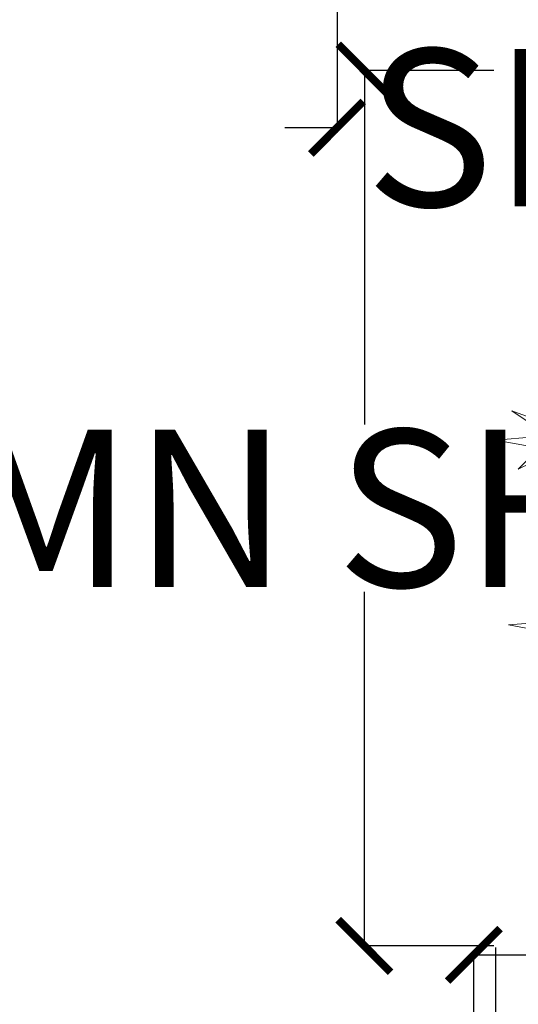
# Model space of a CAD drawing. Units: inches. Extents: x 1704 to 6393, y -157 to 1172.
# Tile 11 of 122: x 1879 to 1898, y 120 to 157. Entities that reach past the tile are written whole.
import ezdxf

# ---------------------------------------------------------------- set-up
doc = ezdxf.new("R2010")
doc.units = ezdxf.units.IN
doc.header["$MEASUREMENT"] = 0
doc.layers.add('A-ANNO-DIMS', color=7, linetype='Continuous', lineweight=13)
doc.layers.add('L-shrub', color=74, linetype='Continuous', lineweight=18)
doc.styles.get("Standard").update_dxf_attribs({"font": 'arial.ttf'})
doc.dimstyles.get("Standard").update_dxf_attribs({"dimtxt": 6, "dimasz": 2, "dimexe": 0.18, "dimexo": 0.0625, "dimgap": 0.09, "dimtad": 0, "dimtih": 1, "dimtoh": 1, "dimdec": 1, "dimzin": 0, "dimdsep": 46, "dimlunit": 3, "dimtxsty": 'Standard', "dimblk": 'ARCHTICK', "dimcen": 0.09, "dimadec": 0, "dimazin": 0, "dimtfac": 1, "dimtdec": 1, "dimtofl": 0, "dimtmove": 0, "dimatfit": 3, "dimfxl": 1, "dimtolj": 1, "dimtzin": 0, "dimarcsym": 0})

# ---------------------------------------------------------------- blocks, each defined once
blk = doc.blocks.new('autumn shrub')
at = {"layer": 'L-shrub'}
for points in [[(-46.17, -236.34), (-38.48, -236.34), (-53.87, -259.4), (-46.17, -238.26)], [(69.26, -238.26), (76.95, -240.18), (73.11, -261.32), (71.18, -238.26)], [(-32.71, -242.11), (-19.24, -255.56), (-26.93, -240.18), (-30.78, -242.11)], [(-40.4, -245.95), (-32.71, -247.87), (-36.55, -269.01), (-38.48, -245.95)]]:
    blk.add_lwpolyline(points, dxfattribs=at)
blk = doc.blocks.new('_ArchTick')
at = {"color": 0, "linetype": 'ByBlock', "const_width": 0.15}
blk.add_lwpolyline([(-0.5, -0.5), (0.5, 0.5)], dxfattribs=at)
blk = doc.blocks.new('*D74')
at = {"layer": 'A-ANNO-DIMS', "color": 0, "lineweight": -2, "transparency": 16777216}
for p, q in [((1890.878, 159.062), (1890.878, 152.884)), ((1931.278, 159.062), (1931.278, 152.884)), ((1890.878, 153.064), (1888.878, 153.064)), ((1931.278, 153.064), (1933.278, 153.064))]:
    blk.add_line(p, q, dxfattribs=at)
at = {"layer": 'Defpoints', "color": 0, "lineweight": -3, "transparency": 16777216}
for p in [(1890.878, 159.124), (1931.278, 159.124), (1931.278, 153.064)]:
    blk.add_point(p, dxfattribs=at)
at = {"layer": 'A-ANNO-DIMS', "color": 0, "lineweight": -2, "transparency": 16777216, "xscale": 2, "yscale": 2, "zscale": 2}
blk.add_blockref('_ArchTick', (1890.878, 153.064), dxfattribs=at)
at = {"layer": 'A-ANNO-DIMS', "color": 0, "lineweight": -2, "transparency": 16777216, "xscale": 2, "yscale": 2, "zscale": 2, "rotation": 180}
blk.add_blockref('_ArchTick', (1931.278, 153.064), dxfattribs=at)
at = {"layer": 'A-ANNO-DIMS', "color": 0, "transparency": 16777216, "insert": (1911.078, 153.064), "char_height": 6, "attachment_point": 5}
blk.add_mtext('\\A1;SHRUB 40', dxfattribs=at)
blk = doc.blocks.new('*D78')
at = {"layer": 'A-ANNO-DIMS', "color": 0, "lineweight": -2, "transparency": 16777216}
for p, q in [((1896.87, 155.246), (1891.743, 155.246)), ((1891.923, 155.246), (1891.923, 141.742)), ((1891.923, 121.849), (1891.923, 135.353)), ((1896.87, 121.849), (1891.743, 121.849))]:
    blk.add_line(p, q, dxfattribs=at)
at = {"layer": 'Defpoints', "color": 0, "lineweight": -3, "transparency": 16777216}
for p in [(1896.932, 155.246), (1891.923, 121.849), (1896.932, 121.849)]:
    blk.add_point(p, dxfattribs=at)
at = {"layer": 'A-ANNO-DIMS', "color": 0, "lineweight": -2, "transparency": 16777216, "xscale": 2, "yscale": 2, "zscale": 2}
for p, rotation in [((1891.923, 155.246), 90), ((1891.923, 121.849), 270)]:
    blk.add_blockref('_ArchTick', p, dxfattribs=dict(at, rotation=rotation))
at = {"layer": 'A-ANNO-DIMS', "color": 0, "transparency": 16777216, "insert": (1891.923, 138.547), "char_height": 6, "attachment_point": 5}
blk.add_mtext('\\A1;AUTUMN SHRUB 33', dxfattribs=at)
blk = doc.blocks.new('*D79')
at = {"layer": 'A-ANNO-DIMS', "color": 0, "lineweight": -2, "transparency": 16777216}
for p, q in [((1896.932, 121.786), (1896.932, 116.659)), ((1930.289, 121.786), (1930.289, 116.659)), ((1896.932, 116.839), (1909.225, 116.839)), ((1930.289, 116.839), (1917.996, 116.839))]:
    blk.add_line(p, q, dxfattribs=at)
at = {"layer": 'Defpoints', "color": 0, "lineweight": -3, "transparency": 16777216}
for p in [(1896.932, 121.849), (1930.289, 121.849), (1930.289, 116.839)]:
    blk.add_point(p, dxfattribs=at)
at = {"layer": 'A-ANNO-DIMS', "color": 0, "lineweight": -2, "transparency": 16777216, "xscale": 2, "yscale": 2, "zscale": 2, "rotation": 180}
blk.add_blockref('_ArchTick', (1896.932, 116.839), dxfattribs=at)
at = {"layer": 'A-ANNO-DIMS', "color": 0, "lineweight": -2, "transparency": 16777216, "xscale": 2, "yscale": 2, "zscale": 2}
blk.add_blockref('_ArchTick', (1930.289, 116.839), dxfattribs=at)
at = {"layer": 'A-ANNO-DIMS', "color": 0, "transparency": 16777216, "insert": (1913.611, 116.839), "char_height": 6, "attachment_point": 5}
blk.add_mtext('\\A1;33', dxfattribs=at)
blk = doc.blocks.new('*D83')
at = {"layer": 'A-ANNO-DIMS', "color": 0, "lineweight": -2, "transparency": 16777216}
for p, q in [((1896.102, 116.575), (1896.102, 121.691)), ((1896.102, 121.511), (1907.632, 121.511)), ((1927.871, 121.511), (1916.342, 121.511)), ((1927.871, 116.575), (1927.871, 121.691))]:
    blk.add_line(p, q, dxfattribs=at)
at = {"layer": 'Defpoints', "color": 0, "lineweight": -3, "transparency": 16777216}
for p in [(1927.871, 121.511), (1896.102, 116.512), (1927.871, 116.512)]:
    blk.add_point(p, dxfattribs=at)
at = {"layer": 'A-ANNO-DIMS', "color": 0, "lineweight": -2, "transparency": 16777216, "xscale": 2, "yscale": 2, "zscale": 2, "rotation": 180}
blk.add_blockref('_ArchTick', (1896.102, 121.511), dxfattribs=at)
at = {"layer": 'A-ANNO-DIMS', "color": 0, "lineweight": -2, "transparency": 16777216, "xscale": 2, "yscale": 2, "zscale": 2}
blk.add_blockref('_ArchTick', (1927.871, 121.511), dxfattribs=at)
at = {"layer": 'A-ANNO-DIMS', "color": 0, "transparency": 16777216, "insert": (1911.987, 121.511), "char_height": 6, "attachment_point": 5}
blk.add_mtext('\\A1;32', dxfattribs=at)
blk = doc.blocks.new('*D93')
at = {"layer": 'A-ANNO-DIMS', "color": 0, "lineweight": -2, "transparency": 16777216}
for p, q in [((2605.286, 895.213), (1829.698, 895.213)), ((1829.878, 895.213), (1829.878, 495.866)), ((1829.878, 90.213), (1829.878, 489.56)), ((2605.286, 90.213), (1829.698, 90.213))]:
    blk.add_line(p, q, dxfattribs=at)
at = {"layer": 'Defpoints', "color": 0, "lineweight": -3, "transparency": 16777216}
for p in [(2605.349, 895.213), (1829.878, 90.213), (2605.349, 90.213)]:
    blk.add_point(p, dxfattribs=at)
at = {"layer": 'A-ANNO-DIMS', "color": 0, "lineweight": -2, "transparency": 16777216, "xscale": 2, "yscale": 2, "zscale": 2}
for p, rotation in [((1829.878, 895.213), 90), ((1829.878, 90.213), 270)]:
    blk.add_blockref('_ArchTick', p, dxfattribs=dict(at, rotation=rotation))
at = {"layer": 'A-ANNO-DIMS', "color": 0, "transparency": 16777216, "insert": (1829.878, 492.713), "char_height": 6, "attachment_point": 5}
blk.add_mtext('\\A1;805', dxfattribs=at)

msp = doc.modelspace()

# ---------------------------------------------------------------- block references
at = {"layer": 'L-shrub', "xscale": 0.0642956299502212, "yscale": 0.0642956299502212, "zscale": 0.0642956299502212, "rotation": 270}
msp.add_blockref('autumn shrub', (1914.228, 138.795), dxfattribs=at)

# ---------------------------------------------------------------- dimensions: what is measured, and where the dimension line sits
at = {"layer": 'A-ANNO-DIMS'}
dim = msp.add_linear_dim(base=(1829.878, 90.213), p1=(2605.349, 895.213), p2=(2605.349, 90.213), angle=90, dimstyle='Standard', override={"dimdec": 0, "dimlfac": 1, "dimrnd": 0, "dimzin": 0, "dimdsep": 46, "dimlunit": 2}, dxfattribs=at)
dim.commit()
dim.dimension.update_dxf_attribs({"geometry": '*D93', "text_midpoint": (1829.878, 492.713)})
dim = msp.add_linear_dim(base=(1931.278, 153.064), p1=(1890.878, 159.124), p2=(1931.278, 159.124), text='SHRUB <>', dimstyle='Standard', override={"dimdec": 0, "dimlfac": 1, "dimrnd": 0, "dimzin": 0, "dimdsep": 46, "dimlunit": 2}, dxfattribs=at)
dim.commit()
dim.dimension.update_dxf_attribs({"geometry": '*D74', "text_midpoint": (1911.078, 153.064)})
dim = msp.add_linear_dim(base=(1891.923, 121.849), p1=(1896.932, 155.246), p2=(1896.932, 121.849), angle=270, text='AUTUMN SHRUB <>', dimstyle='Standard', override={"dimdec": 0, "dimlfac": 1, "dimrnd": 0, "dimzin": 0, "dimdsep": 46, "dimlunit": 2}, dxfattribs=at)
dim.commit()
dim.dimension.update_dxf_attribs({"geometry": '*D78', "text_midpoint": (1891.923, 138.547)})
for base, p1, p2, picture, middle in [((1927.871, 121.511), (1896.102, 116.512), (1927.871, 116.512), '*D83', (1911.987, 121.511)), ((1930.289, 116.839), (1896.932, 121.849), (1930.289, 121.849), '*D79', (1913.611, 116.839))]:
    dim = msp.add_linear_dim(base=base, p1=p1, p2=p2, dimstyle='Standard', override={"dimdec": 0, "dimlfac": 1, "dimrnd": 0, "dimzin": 0, "dimdsep": 46, "dimlunit": 2}, dxfattribs=at)
    dim.commit()
    dim.dimension.update_dxf_attribs({"geometry": picture, "text_midpoint": middle})

doc.saveas('drawing.dxf')
